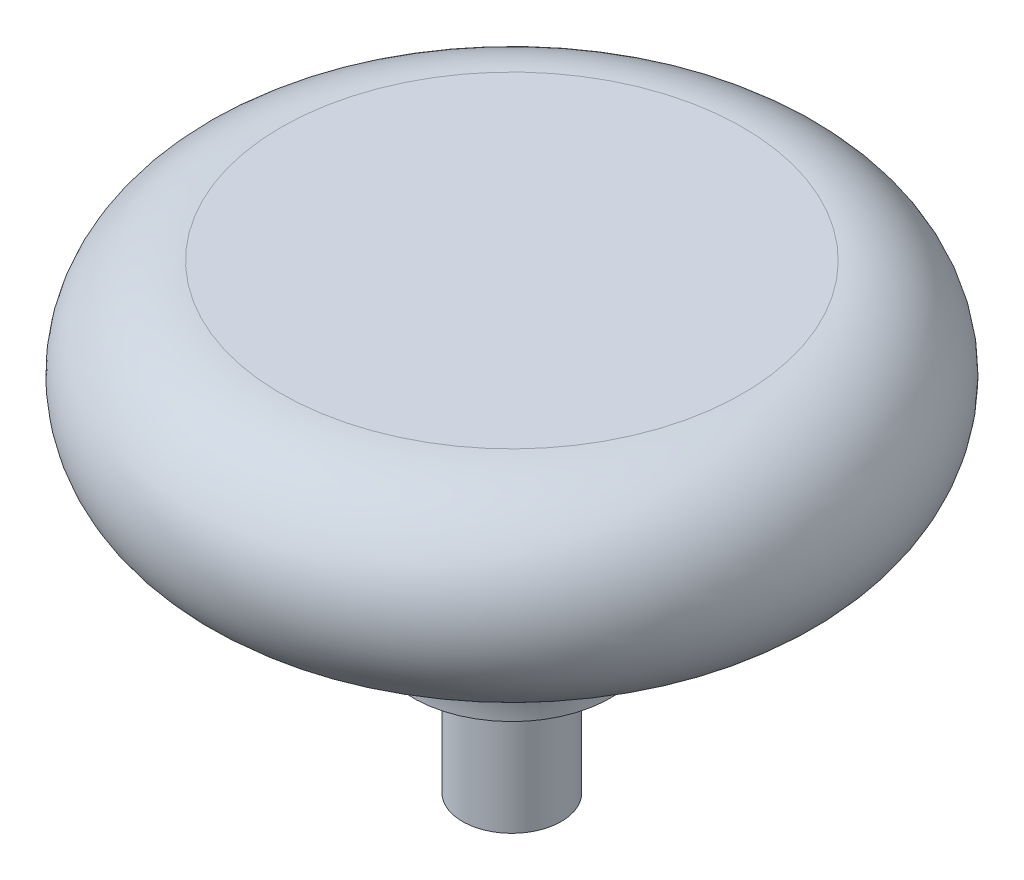
SolidWorks part; units mm, degrees
material "Plain Carbon Steel"
ref_plane "Front Plane" through (0, 0, 0) normal (0, 0, 1) x (1, 0, 0)
ref_plane "Top Plane" through (0, 0, 0) normal (0, 1, 0) x (1, 0, 0)
ref_plane "Right Plane" through (0, 0, 0) normal (1, 0, 0) x (0, 0, -1)
sketch "Knob Profile Sketch" plane through (0, 0, 0) normal (0, 0, 1) x (1, 0, 0)
  line L0 (0, 0) -> (2.38, 0)
  line L1 (2.38, 0) -> (2.38, 6.35)
  line L2 (2.38, 6.35) -> (4.765, 6.35)
  line L3 (11.1179, 22.22) -> (0, 22.22)
  line L4 (0, 22.22) -> (0, 0)
  arc A0 (4.765, 6.35) -> (11.1179, 12.7) centre (11.115, 6.35) cw
  arc A1 (11.1179, 12.7) -> (11.1179, 22.22) centre (11.12, 17.46) ccw
  dimension "D2" = 4.76
  dimension "D3" = 6.35
  dimension "D1" = 11.12
  dimension "D4" = 2.38
  dimension "D5" = 2.385
  dimension "D6" = 22.22
revolve "Knob Body Revolve" add sketch "Knob Profile Sketch" angle 360 about L4
